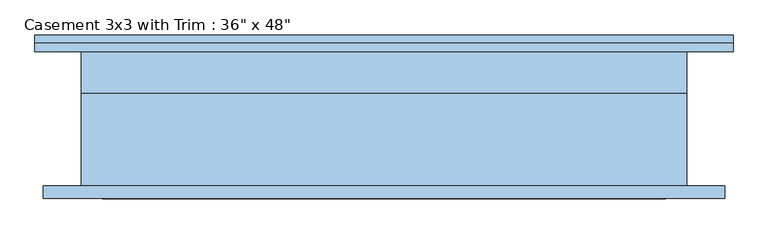
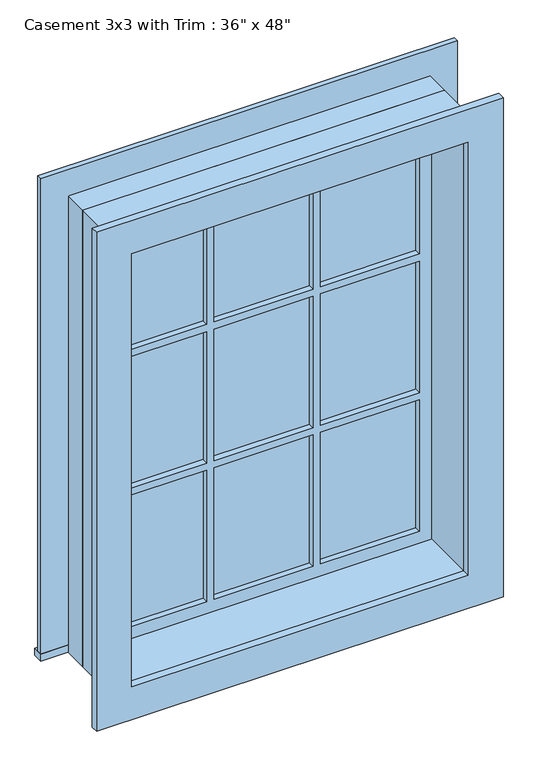
"""IFC4 building model written with IfcOpenShell, lengths in millimetres: window geometry."""

from ifc_helpers import new_model, si_unit, frame, origin, place, context, project, spatial, polyline, outline, extrude, source, transform, mapped, element, save


def window_bd9d39db(model_context):
    return source(origin(), model_context, "Body", "SweptSolid", [
        extrude(outline(polyline([(-527.05, 127.0), (527.05, 127.0), (527.05, 101.6), (-527.05, 101.6), (-527.05, 127.0)])), frame((0.0, 0.0, 1219.2), z_axis=(0.0, 0.0, 1.0), x_axis=(1.0, 0.0, 0.0)), (0.0, 0.0, 1.0), 19.05),
        extrude(outline(polyline([(2419.35, -438.15), (2419.35, 438.15), (1238.25, 438.15), (1238.25, 527.05), (2508.25, 527.05), (2508.25, -527.05), (1238.25, -527.05), (1238.25, -438.15), (2419.35, -438.15)])), frame((0.0, 101.6, 0.0), z_axis=(0.0, 1.0, 0.0), x_axis=(0.0, 0.0, 1.0)), (0.0, 0.0, 1.0), 12.7),
        extrude(outline(polyline([(143.9333333, 66.675), (393.7, 66.675), (393.7, 53.975), (143.9333333, 53.975), (143.9333333, 66.675)])), frame((0.0, 0.0, 2023.5333333), z_axis=(0.0, 0.0, 1.0), x_axis=(1.0, 0.0, 0.0)), (0.0, 0.0, 1.0), 351.3666667),
        extrude(outline(polyline([(-124.8833333, 66.675), (124.8833333, 66.675), (124.8833333, 53.975), (-124.8833333, 53.975), (-124.8833333, 66.675)])), frame((0.0, 0.0, 2023.5333333), z_axis=(0.0, 0.0, 1.0), x_axis=(1.0, 0.0, 0.0)), (0.0, 0.0, 1.0), 351.3666667),
        extrude(outline(polyline([(-393.7, 66.675), (-143.9333333, 66.675), (-143.9333333, 53.975), (-393.7, 53.975), (-393.7, 66.675)])), frame((0.0, 0.0, 2023.5333333), z_axis=(0.0, 0.0, 1.0), x_axis=(1.0, 0.0, 0.0)), (0.0, 0.0, 1.0), 351.3666667),
        extrude(outline(polyline([(-393.7, 66.675), (-143.9333333, 66.675), (-143.9333333, 53.975), (-393.7, 53.975), (-393.7, 66.675)])), frame((0.0, 0.0, 1653.1166667), z_axis=(0.0, 0.0, 1.0), x_axis=(1.0, 0.0, 0.0)), (0.0, 0.0, 1.0), 351.3666667),
        extrude(outline(polyline([(-124.8833333, 66.675), (124.8833333, 66.675), (124.8833333, 53.975), (-124.8833333, 53.975), (-124.8833333, 66.675)])), frame((0.0, 0.0, 1653.1166667), z_axis=(0.0, 0.0, 1.0), x_axis=(1.0, 0.0, 0.0)), (0.0, 0.0, 1.0), 351.3666667),
        extrude(outline(polyline([(143.9333333, 66.675), (393.7, 66.675), (393.7, 53.975), (143.9333333, 53.975), (143.9333333, 66.675)])), frame((0.0, 0.0, 1653.1166667), z_axis=(0.0, 0.0, 1.0), x_axis=(1.0, 0.0, 0.0)), (0.0, 0.0, 1.0), 351.3666667),
        extrude(outline(polyline([(143.9333333, 66.675), (393.7, 66.675), (393.7, 53.975), (143.9333333, 53.975), (143.9333333, 66.675)])), frame((0.0, 0.0, 1282.7), z_axis=(0.0, 0.0, 1.0), x_axis=(1.0, 0.0, 0.0)), (0.0, 0.0, 1.0), 351.3666667),
        extrude(outline(polyline([(-124.8833333, 66.675), (124.8833333, 66.675), (124.8833333, 53.975), (-124.8833333, 53.975), (-124.8833333, 66.675)])), frame((0.0, 0.0, 1282.7), z_axis=(0.0, 0.0, 1.0), x_axis=(1.0, 0.0, 0.0)), (0.0, 0.0, 1.0), 351.3666667),
        extrude(outline(polyline([(-393.7, 66.675), (-143.9333333, 66.675), (-143.9333333, 53.975), (-393.7, 53.975), (-393.7, 66.675)])), frame((0.0, 0.0, 1282.7), z_axis=(0.0, 0.0, 1.0), x_axis=(1.0, 0.0, 0.0)), (0.0, 0.0, 1.0), 351.3666667),
        extrude(outline(polyline([(2495.55, 514.35), (2495.55, -514.35), (1162.05, -514.35), (1162.05, 514.35), (2495.55, 514.35)]), holes=[polyline([(2406.65, 425.45), (1250.95, 425.45), (1250.95, -425.45), (2406.65, -425.45), (2406.65, 425.45)])]), frame((0.0, -120.65, 0.0), z_axis=(0.0, 1.0, 0.0), x_axis=(0.0, 0.0, 1.0)), (0.0, 0.0, 1.0), 19.05),
        extrude(outline(polyline([(2419.35, -438.15), (1238.25, -438.15), (1238.25, 438.15), (2419.35, 438.15), (2419.35, -438.15)]), holes=[polyline([(2374.9, -143.9333333), (2023.5333333, -143.9333333), (2023.5333333, -393.7), (2374.9, -393.7), (2374.9, -143.9333333)]), polyline([(2004.4833333, -143.9333333), (1653.1166667, -143.9333333), (1653.1166667, -393.7), (2004.4833333, -393.7), (2004.4833333, -143.9333333)]), polyline([(1634.0666667, -143.9333333), (1282.7, -143.9333333), (1282.7, -393.7), (1634.0666667, -393.7), (1634.0666667, -143.9333333)]), polyline([(2374.9, 124.8833333), (2023.5333333, 124.8833333), (2023.5333333, -124.8833333), (2374.9, -124.8833333), (2374.9, 124.8833333)]), polyline([(2004.4833333, 124.8833333), (1653.1166667, 124.8833333), (1653.1166667, -124.8833333), (2004.4833333, -124.8833333), (2004.4833333, 124.8833333)]), polyline([(1634.0666667, 124.8833333), (1282.7, 124.8833333), (1282.7, -124.8833333), (1634.0666667, -124.8833333), (1634.0666667, 124.8833333)]), polyline([(2374.9, 393.7), (2023.5333333, 393.7), (2023.5333333, 143.9333333), (2374.9, 143.9333333), (2374.9, 393.7)]), polyline([(2004.4833333, 393.7), (1653.1166667, 393.7), (1653.1166667, 143.9333333), (2004.4833333, 143.9333333), (2004.4833333, 393.7)]), polyline([(1634.0666667, 393.7), (1282.7, 393.7), (1282.7, 143.9333333), (1634.0666667, 143.9333333), (1634.0666667, 393.7)])]), frame((0.0, 38.1, 0.0), z_axis=(0.0, 1.0, 0.0), x_axis=(0.0, 0.0, 1.0)), (0.0, 0.0, 1.0), 44.45),
        extrude(outline(polyline([(2438.4, -457.2), (1219.2, -457.2), (1219.2, 457.2), (2438.4, 457.2), (2438.4, -457.2)]), holes=[polyline([(2406.65, -425.45), (2406.65, 425.45), (1250.95, 425.45), (1250.95, -425.45), (2406.65, -425.45)])]), frame((0.0, -101.6, 0.0), z_axis=(0.0, 1.0, 0.0), x_axis=(0.0, 0.0, 1.0)), (0.0, 0.0, 1.0), 139.7),
        extrude(outline(polyline([(2438.4, 457.2), (2438.4, -457.2), (1219.2, -457.2), (1219.2, 457.2), (2438.4, 457.2)]), holes=[polyline([(2419.35, 438.15), (1238.25, 438.15), (1238.25, -438.15), (2419.35, -438.15), (2419.35, 438.15)])]), frame((0.0, 38.1, 0.0), z_axis=(0.0, 1.0, 0.0), x_axis=(0.0, 0.0, 1.0)), (0.0, 0.0, 1.0), 63.5),
    ])


if __name__ == "__main__":
    model = new_model("IFC4")
    model_context = context("Model", 3, world=origin())
    ifc_project = project(units=[si_unit("LENGTHUNIT", "METRE", prefix="MILLI")], contexts=[model_context])
    site = spatial("IfcSite", under=ifc_project)
    building = spatial("IfcBuilding", under=site)
    placement = place(None, origin())
    window_shape = window_bd9d39db(model_context)
    element("IfcWindow", 1, ObjectType="Casement 3x3 with Trim : 36\" x 48\"", at=placement, inside=building, context=model_context, shape_type="MappedRepresentation", body=[
        mapped(window_shape, transform((0.0, 0.0, 0.0), x_axis=(1.0, 0.0, 0.0), y_axis=(0.0, 1.0, 0.0), z_axis=(0.0, 0.0, 1.0))),
    ])
    save(model, "model.ifc")

# Revit data of these elements
# Type "Casement 3x3 with Trim : 36\" x 48\""
#   Type Mark = "10"
#   Construction Type Id = "GSP4R"
#   Assembly Code = "B2020100"
#   Analytic Construction = "1/8 in Pilkington single glazing"
#   Visual Light Transmittance = 0.9
#   Solar Heat Gain Coefficient = 0.78
#   Heat Transfer Coefficient (U) = 0.6496 BTU/(h·ft²·°F)
#   Height = 4' - 0"
#   Default Sill Height = 4' - 0"
#   Trim Projection - Ext. = 0' - 0 1/2"
#   Trim Projection - Int. = 0' - 0 3/4"
#   Trim Width - Exterior = 0' - 3 1/2"
#   Trim Width - Interior = 0' - 3 1/2"
#   Width = 3' - 0"
#   Window Inset = 0' - 0 3/4"
#   Define Thermal Properties by = 1
#   Glass Pane Material = Glass
#   Sash Material = Sash
#   Trim Exterior Material = Trim
#   Trim Interior Material = Trim
#   Wall Closure = (empty or 0)
# Element 1 (IfcWindow, "Casement 3x3 with Trim : 36\" x 48\"")
#   Materials on its faces: "Sash", "Glass", "Trim"
# Materials
#   "Glass": class "Glass", colour RGB 0 128 192, transparency 0.75, Description = "Soda Lime Glass", Cost = 0
#   "Sash": class "Wood", colour RGB 224 178 126, transparency 0
#   "Trim": class "Wood", colour RGB 224 178 126, transparency 0
